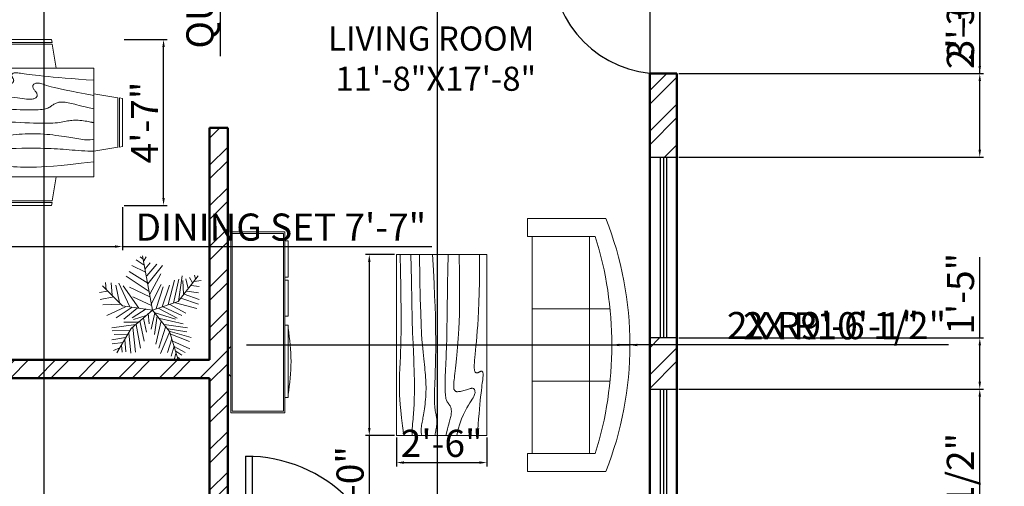
# Model space of a CAD drawing. Units: inches. Extents: x 635 to 1184, y 1837 to 2697.
# Tile 4 of 6: x 857 to 1184, y 2201 to 2356. Entities that reach past the tile are written whole.
import ezdxf

# ---------------------------------------------------------------- set-up
doc = ezdxf.new("R2010")
doc.units = ezdxf.units.IN
for name, color, linetype, lineweight in [('A-ANNO-DIMS', 2, 'Continuous', 18), ('A-AREA-IDEN', 7, 'Continuous', 25), ('A-DOOR', 4, 'Continuous', 25), ('A-FURN', 8, 'Continuous', 18), ('A-GLAZ', 244, 'Continuous', 25), ('A-WALL', 7, 'Continuous', 50), ('A-WALL-PATT', 252, 'Continuous', 13), ('L-PLNT', 94, 'Continuous', 13)]:
    doc.layers.add(name, color=color, linetype=linetype, lineweight=lineweight)
doc.styles.get("Standard").update_dxf_attribs({"font": 'arial.ttf'})
doc.dimstyles.new('ISO-25', dxfattribs={"dimtxt": 9, "dimasz": 2.5, "dimexe": 1.25, "dimexo": 0.625, "dimtad": 1, "dimlunit": 3, "dimtxsty": 'Standard', "dimcen": 2.5, "dimadec": 0, "dimazin": 0, "dimtfac": 1, "dimtmove": 0, "dimatfit": 3, "dimfxl": 1, "dimarcsym": 0})

# ---------------------------------------------------------------- blocks, each defined once
blk = doc.blocks.new('*U3')
for p, q in [((0, 0), (0, -6)), ((40, 0), (40, -6))]:
    blk.add_line(p, q)
blk.add_lwpolyline([(0, 0), (0, 40), (1.75, 40), (1.75, 0)], close=True)
blk.add_arc((0, 0), 40, 0, 90)
blk = doc.blocks.new('*U4')
for p, q in [((0, 0), (0, -6)), ((-40, 0), (-40, -6))]:
    blk.add_line(p, q)
blk.add_lwpolyline([(0, 0), (0, 40), (-1.75, 40), (-1.75, 0)], close=True)
blk.add_arc((0, 0), 40, 90, 180)
blk = doc.blocks.new('Dining Set - 36 x 72 in.')
for p, q in [((-22, 27.5), (-22.1562, 26.50042)), ((-5.8416, 26.5), (-22.1534, 26.5)), ((-22, 27.5), (-6, 27.5)), ((-5.8437, 26.49966), (-6, 27.5)), ((6, 27.5), (5.8438, 26.50042)), ((22.1584, 26.5), (5.8466, 26.5)), ((6, 27.5), (22, 27.5)), ((22.1563, 26.49966), (22, 27.5)), ((-22.2343, 26.00059), (-23.4847, 17.99762)), ((-22.2304, 26), (-5.7608, 26)), ((-4.5152, 17.99762), (-5.7655, 25.99926)), ((5.7657, 26.00059), (4.5153, 17.99762)), ((5.7696, 26), (22.2392, 26)), ((23.4848, 17.99762), (22.2345, 25.99926)), ((36, 18), (-36, 18)), ((-36, 18), (-36, -18)), ((36, -18), (36, 18)), ((-45.5, 8), (-44.5004, 8.15617)), ((-45.5, 8), (-45.5, -8)), ((-44.5, -8.15843), (-44.5, 8.15338)), ((-44.0006, 8.23428), (-35.9976, 9.48474)), ((-44, 8.23041), (-44, -8.23915)), ((44.0006, 8.23428), (35.9976, 9.48474)), ((44, 8.23041), (44, -8.23915)), ((44.5, -8.15843), (44.5, 8.15338)), ((45.5, 8), (44.5005, 8.15617)), ((45.5, 8), (45.5, -8)), ((-44.4997, -8.15631), (-45.5, -8)), ((-35.9976, -9.48476), (-43.9993, -8.2345)), ((35.9976, -9.48476), (43.9993, -8.2345)), ((44.4997, -8.15631), (45.5, -8)), ((-36, -18), (36, -18)), ((-22.2343, -26.0006), (-23.4847, -17.99762)), ((-4.5152, -17.99762), (-5.7655, -25.99928)), ((5.7657, -26.0006), (4.5153, -17.99762)), ((23.4848, -17.99762), (22.2345, -25.99928)), ((-22.2304, -26), (-5.7608, -26)), ((5.7696, -26), (22.2392, -26)), ((-22, -27.5), (-22.1562, -26.50044)), ((-5.8416, -26.5), (-22.1534, -26.5)), ((-22, -27.5), (-6, -27.5)), ((-5.8437, -26.49967), (-6, -27.5)), ((6, -27.5), (5.8438, -26.50044)), ((22.1584, -26.5), (5.8466, -26.5)), ((6, -27.5), (22, -27.5)), ((22.1563, -26.49967), (22, -27.5))]:
    blk.add_line(p, q)
for points in [[(-36, 15), (-31.1772, 14.97754), (-26.8079, 14.91406), (-22.8538, 14.81543), (-19.276, 14.6875), (-16.0362, 14.53613), (-13.0957, 14.36718), (-10.4159, 14.18652), (-7.9583, 14), (-5.6904, 13.81315), (-3.6035, 13.63021), (-1.6954, 13.45508), (0.0365, 13.29166), (1.5945, 13.14388), (2.9811, 13.01562), (4.1988, 12.9108), (5.25, 12.83333), (6.1393, 12.78613), (6.8802, 12.76823), (7.4883, 12.77767), (7.9792, 12.8125), (8.3685, 12.87077), (8.6719, 12.95052), (8.9049, 13.0498), (9.0833, 13.16666), (9.2205, 13.29899), (9.3216, 13.44401), (9.3895, 13.59879), (9.4271, 13.76041), (9.4373, 13.92594), (9.4232, 14.09245), (9.3875, 14.257), (9.3333, 14.41666), (9.2638, 14.56917), (9.1836, 14.71484), (9.0975, 14.85465), (9.0104, 14.98958), (8.9272, 15.1206), (8.8529, 15.2487), (8.7922, 15.37483), (8.75, 15.5), (8.7305, 15.62467), (8.7344, 15.74739), (8.7617, 15.86621), (8.8125, 15.97916), (8.8867, 16.08431), (8.9844, 16.17968), (9.1055, 16.26334), (9.25, 16.33333), (9.4189, 16.38802), (9.6172, 16.42708), (9.8506, 16.45052), (10.125, 16.45833), (10.4463, 16.45052), (10.8203, 16.42708), (11.2529, 16.38802), (11.75, 16.33333), (12.3184, 16.26318), (12.9694, 16.17838), (13.7151, 16.07991), (14.5677, 15.96875), (15.5395, 15.84586), (16.6426, 15.71224), (17.8893, 15.56884), (19.2917, 15.41666), (20.859, 15.25667), (22.5879, 15.08984), (24.4721, 14.91715), (26.5052, 14.73958), (28.6809, 14.5581), (30.9929, 14.3737), (33.4347, 14.18733), (36, 14)], [(-36, 10), (-28.9766, 10.14274), (-23.1725, 10.20442), (-18.4241, 10.19775), (-14.5677, 10.13541), (-11.4399, 10.03011), (-8.877, 9.89453), (-6.7154, 9.74137), (-4.7917, 9.58333), (-2.9698, 9.43082), (-1.2246, 9.28515), (0.4415, 9.14534), (2.026, 9.01041), (3.5266, 8.87939), (4.9408, 8.7513), (6.266, 8.62516), (7.5, 8.5), (8.6411, 8.37549), (9.6914, 8.2539), (10.6538, 8.13818), (11.5312, 8.03125), (12.3267, 7.93603), (13.043, 7.85547), (13.6831, 7.79248), (14.25, 7.75), (14.7471, 7.7303), (15.1797, 7.73307), (15.5537, 7.75732), (15.875, 7.80208), (16.1494, 7.86637), (16.3828, 7.94922), (16.5811, 8.04964), (16.75, 8.16666), (16.8944, 8.29915), (17.0143, 8.44531), (17.1089, 8.60319), (17.1771, 8.77083), (17.218, 8.94629), (17.2305, 9.1276), (17.2137, 9.31282), (17.1667, 9.5), (17.0895, 9.6875), (16.987, 9.875), (16.8649, 10.0625), (16.7292, 10.25), (16.5856, 10.4375), (16.4401, 10.625), (16.2985, 10.8125), (16.1667, 11), (16.05, 11.18733), (15.9518, 11.3737), (15.8752, 11.5581), (15.8229, 11.73958), (15.798, 11.91715), (15.8034, 12.08984), (15.842, 12.25667), (15.9167, 12.41666), (16.0295, 12.56836), (16.1784, 12.70833), (16.3605, 12.83268), (16.5729, 12.9375), (16.8127, 13.01888), (17.0768, 13.07291), (17.3625, 13.0957), (17.6667, 13.08333), (17.9894, 13.03312), (18.3418, 12.94726), (18.7382, 12.82918), (19.1927, 12.68229), (19.7195, 12.51001), (20.3327, 12.31575), (21.0465, 12.10294), (21.875, 11.875), (22.8357, 11.63354), (23.959, 11.37304), (25.2786, 11.08618), (26.8282, 10.76562), (28.6414, 10.40405), (30.752, 9.99414), (33.1936, 9.52856), (36, 9)], [(-36, 5.5), (-30.7157, 5.3348), (-26.069, 5.20963), (-21.9946, 5.11767), (-18.4271, 5.05208), (-15.3009, 5.00602), (-12.5508, 4.97265), (-10.1112, 4.94515), (-7.9167, 4.91666), (-5.909, 4.88167), (-4.0586, 4.83984), (-2.3429, 4.79215), (-0.7396, 4.73958), (0.7739, 4.6831), (2.22, 4.6237), (3.6213, 4.56233), (5, 4.5), (6.373, 4.43782), (7.7344, 4.3776), (9.0723, 4.32129), (10.375, 4.27083), (11.6309, 4.22819), (12.8281, 4.19531), (13.9551, 4.17415), (15, 4.16666), (15.954, 4.17448), (16.819, 4.19791), (17.6001, 4.23698), (18.3021, 4.29166), (18.9299, 4.36198), (19.4883, 4.44791), (19.9823, 4.54948), (20.4167, 4.66666), (20.7969, 4.79899), (21.1302, 4.94401), (21.4245, 5.09879), (21.6875, 5.26041), (21.9271, 5.42594), (22.1511, 5.59245), (22.3672, 5.757), (22.5834, 5.91666), (22.8065, 6.06868), (23.0404, 6.21093), (23.2879, 6.34147), (23.5521, 6.45833), (23.8358, 6.55957), (24.142, 6.64323), (24.4735, 6.70735), (24.8334, 6.75), (25.2235, 6.76969), (25.642, 6.76692), (26.0858, 6.74267), (26.5521, 6.69791), (27.0379, 6.63362), (27.5404, 6.55078), (28.0565, 6.45036), (28.5834, 6.33333), (29.1242, 6.19987), (29.7071, 6.04687), (30.3661, 5.87044), (31.1354, 5.66666), (32.0493, 5.43164), (33.142, 5.16146), (34.4475, 4.85221), (36, 4.5)], [(-36, -1), (-30.7915, -0.6591), (-26.0195, -0.38216), (-21.6519, -0.16284), (-17.6563, 0.00521), (-14.0005, 0.12833), (-10.6523, 0.21289), (-7.5796, 0.26522), (-4.75, 0.29166), (-2.134, 0.29793), (0.2878, 0.28711), (2.5317, 0.26163), (4.6146, 0.22396), (6.5529, 0.17651), (8.3633, 0.12174), (10.0623, 0.06209), (11.6667, 0), (13.1899, -0.06201), (14.6341, -0.1211), (15.9982, -0.17432), (17.2813, -0.21875), (18.4823, -0.25147), (19.6003, -0.26953), (20.6343, -0.27002), (21.5834, -0.25), (22.4481, -0.20768), (23.2357, -0.14584), (23.9549, -0.06836), (24.6146, 0.02083), (25.2235, 0.11784), (25.7904, 0.21875), (26.3241, 0.31966), (26.8334, 0.41666), (27.3265, 0.50618), (27.8099, 0.58593), (28.2894, 0.65397), (28.7709, 0.70833), (29.2601, 0.74707), (29.763, 0.76823), (30.2855, 0.76985), (30.8334, 0.75), (31.4088, 0.70784), (31.9994, 0.64713), (32.589, 0.57275), (33.1615, 0.48958), (33.7008, 0.4025), (34.1908, 0.3164), (34.6153, 0.23616), (34.9584, 0.16666), (35.2099, 0.11165), (35.3848, 0.07031), (35.504, 0.04069), (35.5886, 0.02083), (35.6594, 0.00879), (35.7377, 0.0026), (35.8442, 0.00032), (36, 0)], [(-36, -6.5), (-27.1843, -6.31267), (-20.084, -6.1263), (-14.469, -5.9419), (-10.1094, -5.76042), (-6.7752, -5.58285), (-4.2363, -5.41016), (-2.2629, -5.24333), (-0.625, -5.08334), (0.8708, -4.93099), (2.2715, -4.78646), (3.5872, -4.64974), (4.8281, -4.52084), (6.0046, -4.39974), (7.127, -4.28646), (8.2053, -4.18099), (9.25, -4.08334), (10.2705, -3.99382), (11.2734, -3.91407), (12.2647, -3.84603), (13.25, -3.79167), (14.2354, -3.75293), (15.2266, -3.73177), (16.2295, -3.73015), (17.25, -3.75), (18.2912, -3.79248), (19.3451, -3.85547), (20.4009, -3.93604), (21.4479, -4.03125), (22.4754, -4.13819), (23.4727, -4.25391), (24.4289, -4.37549), (25.3334, -4.5), (26.1785, -4.62492), (26.9694, -4.74935), (27.7145, -4.87281), (28.4219, -4.99479), (29.1, -5.11483), (29.7572, -5.23242), (30.4016, -5.34709), (31.0417, -5.45834), (31.6837, -5.56437), (32.3262, -5.65821), (32.9658, -5.73153), (33.599, -5.77604), (34.2224, -5.78345), (34.8327, -5.74545), (35.4264, -5.65373), (36, -5.5)], [(-36, -10), (-26.4022, -9.81299), (-18.4675, -9.62891), (-11.9839, -9.45069), (-6.7396, -9.28125), (-2.5226, -9.12354), (0.8789, -8.98047), (3.6769, -8.85498), (6.0833, -8.75), (8.2767, -8.66765), (10.3021, -8.60677), (12.1712, -8.56543), (13.8958, -8.54167), (15.4876, -8.53353), (16.9583, -8.53907), (18.3197, -8.55632), (19.5834, -8.58334), (20.7616, -8.61841), (21.8685, -8.66081), (22.9188, -8.71004), (23.9271, -8.76563), (24.9081, -8.82707), (25.8763, -8.89388), (26.8465, -8.96558), (27.8334, -9.04167), (28.8474, -9.12118), (29.8828, -9.20117), (30.93, -9.27824), (31.9792, -9.34896), (33.0205, -9.40991), (34.0443, -9.45768), (35.0407, -9.48885), (36, -9.5)], [(-36, -14.5), (-30.0881, -14.33513), (-25.0332, -14.21224), (-20.7312, -14.12647), (-17.0781, -14.07292), (-13.97, -14.04671), (-11.3027, -14.04297), (-8.9724, -14.05681), (-6.875, -14.08334), (-4.9224, -14.11833), (-3.0905, -14.16016), (-1.3709, -14.20785), (0.2448, -14.26042), (1.7647, -14.3169), (3.1973, -14.3763), (4.5507, -14.43767), (5.8333, -14.5), (7.0554, -14.5621), (8.235, -14.62175), (9.3922, -14.67652), (10.5469, -14.72396), (11.7192, -14.76164), (12.929, -14.78711), (14.1965, -14.79794), (15.5417, -14.79167), (16.9933, -14.76424), (18.6152, -14.70508), (20.4804, -14.60197), (22.6615, -14.44271), (25.2312, -14.21509), (28.2624, -13.9069), (31.8277, -13.50594), (36, -13)]]:
    blk.add_lwpolyline(points)
blk = doc.blocks.new('Sofa - Roundback 7 ft.')
for p, q in [((-12.00002, -32.4421), (-12.00003, -6.5971)), ((11.99997, -32.4421), (11.99998, -6.5971)), ((-36.000027, -34), (-36.000027, -11.4696)), ((35.99998, -34), (35.99998, -11.4696)), ((-35.999844, -13.3819), (35.9998, -13.3819)), ((-36.000027, -32.4421), (35.99998, -32.4421))]:
    blk.add_line(p, q)
for points in [[(-36.000027, -34), (-42.000027, -34), (-42.000027, -8)], [(41.99998, -8), (41.99998, -34), (35.99998, -34)]]:
    blk.add_lwpolyline(points)
for centre, radius, start, end in [((0, -114.25), 114.25, 68.43141, 111.5686), ((-0.00001, -127.1968), 121.1968, 72.72033, 107.2797)]:
    blk.add_arc(centre, radius, start, end)
blk = doc.blocks.new('Table - Rectangular Woodgrain 60 x 30 in.')
for p, q in [((0, 0), (0, -30)), ((60, 0), (0, 0)), ((60, -30), (60, 0)), ((0, -30), (60, -30))]:
    blk.add_line(p, q)
for points in [[(0, -2.4), (4.8155, -2.418), (9.0302, -2.4688), (12.709, -2.5477), (15.9167, -2.65), (18.7181, -2.7711), (21.1781, -2.9063), (23.3616, -3.0508), (25.3333, -3.2), (27.1477, -3.3495), (28.8172, -3.4958), (30.3437, -3.636), (31.7291, -3.7667), (32.9756, -3.8849), (34.0849, -3.9875), (35.059, -4.0714), (35.9, -4.1334), (36.6114, -4.1711), (37.2041, -4.1854), (37.6906, -4.1779), (38.0833, -4.15), (38.3948, -4.1034), (38.6375, -4.0396), (38.8239, -3.9602), (38.9666, -3.8667), (39.0764, -3.7608), (39.1573, -3.6448), (39.2116, -3.521), (39.2416, -3.3917), (39.2498, -3.2593), (39.2385, -3.1261), (39.21, -2.9944), (39.1666, -2.8667), (39.111, -2.7447), (39.0468, -2.6281), (38.978, -2.5163), (38.9083, -2.4083), (38.8418, -2.3035), (38.7823, -2.201), (38.7337, -2.1001), (38.7, -2), (38.6844, -1.9003), (38.6875, -1.8021), (38.7094, -1.707), (38.75, -1.6167), (38.8094, -1.5326), (38.8875, -1.4563), (38.9844, -1.3893), (39.1, -1.3333), (39.2351, -1.2896), (39.3937, -1.2583), (39.5804, -1.2396), (39.8, -1.2333), (40.057, -1.2396), (40.3562, -1.2583), (40.7023, -1.2896), (41.1, -1.3333), (41.5547, -1.3895), (42.0755, -1.4573), (42.6721, -1.5361), (43.3542, -1.625), (44.1316, -1.7233), (45.014, -1.8302), (46.0114, -1.9449), (47.1333, -2.0667), (48.3862, -2.1947), (49.7625, -2.3281), (51.2513, -2.4663), (52.8416, -2.6083), (54.5226, -2.7535), (56.2833, -2.9011), (58.1127, -3.0501), (60, -3.2)], [(0, -9.2), (6.5759, -9.0858), (11.9385, -9.0365), (16.2527, -9.0418), (19.6833, -9.0917), (22.3952, -9.1759), (24.5531, -9.2844), (26.322, -9.4069), (27.8666, -9.5333), (29.3241, -9.6553), (30.7203, -9.7719), (32.0532, -9.8837), (33.3208, -9.9917), (34.5213, -10.0965), (35.6526, -10.199), (36.7128, -10.2999), (37.7, -10.4), (38.6129, -10.4996), (39.4531, -10.5969), (40.223, -10.6895), (40.925, -10.775), (41.5613, -10.8512), (42.1344, -10.9156), (42.6465, -10.966), (43.1, -11), (43.4976, -11.0158), (43.8437, -11.0136), (44.143, -10.9942), (44.4, -10.9583), (44.6195, -10.9069), (44.8062, -10.8406), (44.9648, -10.7603), (45.1, -10.6667), (45.2155, -10.5598), (45.3114, -10.4365), (45.3871, -10.2929), (45.4416, -10.125), (45.4743, -9.929), (45.4844, -9.7011), (45.4709, -9.4371), (45.4333, -9.1333), (45.3716, -8.7883), (45.2896, -8.4104), (45.1919, -8.0107), (45.0833, -7.6), (44.9685, -7.1893), (44.8521, -6.7896), (44.7388, -6.4117), (44.6333, -6.0667), (44.54, -5.7628), (44.4614, -5.4979), (44.4001, -5.2675), (44.3583, -5.0667), (44.3384, -4.8909), (44.3427, -4.7354), (44.3736, -4.5956), (44.4333, -4.4667), (44.5236, -4.3453), (44.6427, -4.2333), (44.7884, -4.1339), (44.9583, -4.05), (45.1501, -3.9849), (45.3614, -3.9417), (45.59, -3.9234), (45.8333, -3.9333), (46.0915, -3.9749), (46.3734, -4.0531), (46.6906, -4.1736), (47.0542, -4.3417), (47.4756, -4.5629), (47.9661, -4.8427), (48.5372, -5.1866), (49.2, -5.6), (49.9676, -6.0844), (50.8594, -6.625), (51.8965, -7.2031), (53.1, -7.8), (54.491, -8.3969), (56.0906, -8.975), (57.9199, -9.5156), (60, -10)], [(0, -12.8), (5.1847, -12.9322), (9.6213, -13.0323), (13.3963, -13.1059), (16.5958, -13.1583), (19.3063, -13.1952), (21.614, -13.2219), (23.6054, -13.2439), (25.3666, -13.2667), (26.9728, -13.2947), (28.4531, -13.3281), (29.8256, -13.3663), (31.1083, -13.4083), (32.3191, -13.4535), (33.476, -13.501), (34.597, -13.5501), (35.7, -13.6), (36.7984, -13.6497), (37.8875, -13.6979), (38.9578, -13.743), (40, -13.7833), (41.0047, -13.8174), (41.9625, -13.8438), (42.864, -13.8607), (43.7, -13.8667), (44.4631, -13.8604), (45.1552, -13.8417), (45.7801, -13.8104), (46.3416, -13.7667), (46.8439, -13.7104), (47.2906, -13.6417), (47.6858, -13.5604), (48.0333, -13.4667), (48.3375, -13.3608), (48.6042, -13.2448), (48.8396, -13.121), (49.05, -12.9917), (49.2417, -12.8593), (49.4208, -12.7261), (49.5937, -12.5944), (49.7667, -12.4667), (49.9452, -12.3451), (50.1323, -12.2313), (50.3303, -12.1268), (50.5416, -12.0333), (50.7686, -11.9524), (51.0135, -11.8854), (51.2788, -11.8341), (51.5666, -11.8), (51.8785, -11.7843), (52.2116, -11.7865), (52.562, -11.8059), (52.926, -11.8417), (53.2998, -11.8931), (53.6795, -11.9594), (54.0614, -12.0397), (54.4416, -12.1333), (54.8223, -12.2401), (55.2293, -12.3625), (55.6942, -12.5037), (56.2489, -12.6667), (56.9251, -12.8547), (57.7545, -13.0708), (58.7689, -13.3182), (60, -13.6)], [(0, -18), (5.124, -17.7273), (9.6609, -17.5057), (13.6705, -17.3303), (17.2125, -17.1958), (20.3467, -17.0973), (23.1328, -17.0297), (25.6307, -16.9878), (27.9, -16.9667), (29.9928, -16.9617), (31.9302, -16.9703), (33.7254, -16.9907), (35.3917, -17.0208), (36.9423, -17.0588), (38.3906, -17.1026), (39.7499, -17.1503), (41.0333, -17.2), (42.2519, -17.2496), (43.4073, -17.2969), (44.4986, -17.3395), (45.525, -17.375), (46.4858, -17.4012), (47.3802, -17.4156), (48.2074, -17.416), (48.9667, -17.4), (49.6583, -17.3662), (50.2872, -17.3167), (50.8595, -17.2547), (51.3812, -17.1833), (51.8584, -17.1057), (52.2971, -17.025), (52.7034, -16.9443), (53.0833, -16.8667), (53.443, -16.7951), (53.789, -16.7313), (54.128, -16.6768), (54.4666, -16.6334), (54.8115, -16.6024), (55.1693, -16.5854), (55.5465, -16.5841), (55.95, -16.6), (56.3828, -16.6337), (56.8346, -16.6823), (57.2915, -16.7418), (57.7396, -16.8084), (58.165, -16.878), (58.5539, -16.9469), (58.8924, -17.0111), (59.1666, -17.0667), (59.3679, -17.1107), (59.5078, -17.1438), (59.6032, -17.1675), (59.6708, -17.1833), (59.7275, -17.193), (59.7901, -17.1979), (59.8753, -17.1998), (60, -17.2)], [(0, -22.4), (8.0098, -22.2501), (14.4094, -22.1011), (19.4168, -21.9535), (23.25, -21.8083), (26.1269, -21.6663), (28.2656, -21.5281), (29.884, -21.3947), (31.2, -21.2667), (32.3967, -21.1448), (33.5172, -21.0292), (34.5697, -20.9198), (35.5625, -20.8167), (36.5037, -20.7198), (37.4015, -20.6292), (38.2642, -20.5448), (39.1, -20.4667), (39.9164, -20.3951), (40.7187, -20.3313), (41.5117, -20.2768), (42.3, -20.2333), (43.0883, -20.2024), (43.8812, -20.1854), (44.6836, -20.1841), (45.5, -20.2), (46.3328, -20.234), (47.1747, -20.2844), (48.0163, -20.3488), (48.8479, -20.425), (49.66, -20.5106), (50.4429, -20.6031), (51.1872, -20.7004), (51.8833, -20.8), (52.5246, -20.8999), (53.1166, -20.9995), (53.6681, -21.0983), (54.1875, -21.1958), (54.6834, -21.2919), (55.1646, -21.3859), (55.6394, -21.4777), (56.1167, -21.5667), (56.6028, -21.6515), (57.0961, -21.7266), (57.5929, -21.7852), (58.0896, -21.8208), (58.5823, -21.8268), (59.0674, -21.7964), (59.5412, -21.723), (60, -21.6)], [(0, -25.2), (8.6355, -25.0504), (15.7026, -24.9031), (21.4049, -24.7606), (25.9458, -24.625), (29.529, -24.4988), (32.3578, -24.3844), (34.6359, -24.284), (36.5667, -24.2), (38.3213, -24.1341), (39.9417, -24.0854), (41.437, -24.0523), (42.8167, -24.0333), (44.0901, -24.0268), (45.2667, -24.0313), (46.3557, -24.0451), (47.3667, -24.0667), (48.309, -24.0947), (49.1928, -24.1287), (50.0284, -24.168), (50.826, -24.2125), (51.5959, -24.2617), (52.3483, -24.3151), (53.0935, -24.3725), (53.8417, -24.4334), (54.6009, -24.497), (55.3699, -24.561), (56.1454, -24.6226), (56.9239, -24.6792), (57.7021, -24.7279), (58.4764, -24.7662), (59.2435, -24.7911), (60, -24.8)], [(0, -28.8), (5.6867, -28.6681), (10.45, -28.5698), (14.407, -28.5012), (17.675, -28.4584), (20.3711, -28.4374), (22.6125, -28.4344), (24.5164, -28.4455), (26.2, -28.4667), (27.762, -28.4947), (29.2276, -28.5281), (30.6033, -28.5663), (31.8958, -28.6084), (33.1118, -28.6535), (34.2578, -28.7011), (35.3405, -28.7501), (36.3666, -28.8), (37.3443, -28.8497), (38.288, -28.8974), (39.2137, -28.9412), (40.1375, -28.9792), (41.0753, -29.0093), (42.0432, -29.0297), (43.0572, -29.0384), (44.1333, -29.0333), (45.2936, -29.0114), (46.5843, -28.9641), (48.0579, -28.8816), (49.7666, -28.7542), (51.7629, -28.5721), (54.0989, -28.3255), (56.8272, -28.0048), (60, -27.6)]]:
    blk.add_lwpolyline(points)
blk = doc.blocks.new('Entertainment Center')
for p, q in [((-4, 0), (-5, -1)), ((4, 0), (-4, 0)), ((5, -1), (4, 0)), ((-17, -19), (-17, -1)), ((-17, -1), (43, -1)), ((-16.5, -18.5), (-16.5, -1.5)), ((-16.5, -1.5), (42.5, -1.5)), ((42.5, -1.5), (42.5, -18.5)), ((43, -1), (43, -19)), ((43, -19), (-17, -19)), ((42.5, -18.5), (-16.5, -18.5)), ((-12, -20), (-12, -19)), ((12, -19), (12, -20)), ((15, -20), (15, -19)), ((27, -19), (27, -20)), ((28, -20), (28, -19)), ((40, -19), (40, -20)), ((12, -20), (-12, -20)), ((27, -20), (15, -20)), ((40, -20), (28, -20))]:
    blk.add_line(p, q)
blk.add_arc((0, 40), 61, 259.6111, 280.3889)
blk = doc.blocks.new('*U15')
for p, q in [((-8.737, 47.138), (-17.069, 52.711)), ((-10.186, 53.64), (-13.084, 55.962)), ((0, 0), (-10.5, 57)), ((-9.099, 51.782), (-6.563, 55.962)), ((-7.288, 39.707), (-21.778, 46.673)), ((-7.65, 43.423), (-2.578, 49.46)), ((-5.839, 35.992), (4.667, 48.067)), ((-5.114, 27.632), (10.463, 46.673)), ((-3.665, 19.273), (-27.574, 35.527)), ((-5.114, 28.097), (-24.676, 40.636)), ((-2.941, 16.486), (8.652, 37.85)), ((16.259, 5.805), (23.142, 31.348)), ((22.055, 7.198), (27.489, 32.277)), ((27, 9), (48, 36)), ((27.127, 9.056), (31.112, 35.992)), ((35.096, 32.741), (37.27, 22.524)), ((38.719, 34.134), (41.979, 28.561)), ((44.153, 36.456), (45.239, 32.741)), ((-31.5, 4.5), (-52.5, 25.5)), ((-48.585, 21.131), (-49.309, 29.026)), ((-43.513, 28.561), (-42.427, 15.558)), ((-38.442, 26.239), (-34.819, 7.663)), ((-35.544, 28.097), (-24.314, 3.947)), ((-14.533, 2.09), (-30.834, 25.31)), ((-24.314, 23.917), (-2.941, 13.7)), ((-1.129, 6.734), (9.014, 26.704)), ((3.942, 1.625), (11.187, 24.381)), ((10.101, 3.483), (17.708, 26.239)), ((31.836, 30.883), (32.561, 16.486)), ((40.53, 25.775), (48.862, 24.846)), ((43.791, 29.954), (51.036, 30.883)), ((-47.498, 19.737), (-55.83, 18.344)), ((-40.615, 13.7), (-55.105, 10.913)), ((-20.691, 13.7), (-1.129, 4.876)), ((29.662, 12.307), (48.137, 6.269)), ((33.285, 16.486), (48.862, 10.913)), ((36.183, 19.737), (48.137, 17.88)), ((-33.37, 6.269), (-52.207, 5.34)), ((-28.299, 3.483), (-47.86, -5.805)), ((-21.416, 3.018), (-38.079, -8.128)), ((0, 0), (-31.5, 4.5)), ((-15.982, 2.09), (-30.11, -9.521)), ((0, 0), (-22.5, -19.5)), ((-6.563, 1.161), (-21.416, -8.128)), ((0, 0), (27, 9)), ((0, 0), (18, -22.5)), ((6.478, 1.625), (26.04, -8.592)), ((11.187, 3.483), (30.749, -5.805)), ((18.07, 5.805), (35.096, -3.483)), ((24.229, 7.663), (46.688, 1.625)), ((-6.563, -5.805), (-19.967, -9.985)), ((-9.461, -8.592), (-6.201, -23.453)), ((-4.752, -3.483), (-3.665, -14.629)), ((2.493, -3.019), (-1.491, -20.202)), ((1.769, -2.555), (24.229, -9.521)), ((5.029, -6.27), (2.131, -25.775)), ((7.565, -9.056), (32.198, -14.629)), ((-17.431, -15.094), (-42.789, -18.809)), ((-22.5, -19.5), (-37.5, -45)), ((-15.257, -12.772), (-30.11, -12.772)), ((-20.691, -18.345), (-17.793, -44.352)), ((-17.069, -15.094), (-12.721, -40.172)), ((-13.446, -11.378), (-8.737, -32.741)), ((9.014, -11.378), (3.58, -35.992)), ((14.085, -16.951), (6.478, -40.172)), ((12.274, -15.094), (36.907, -18.809)), ((16.259, -19.738), (36.183, -22.989)), ((-28.299, -29.026), (-42.789, -31.348)), ((-24.314, -21.596), (-42.427, -22.06)), ((-26.849, -26.24), (-40.253, -25.775)), ((-29.023, -30.884), (-27.936, -43.887)), ((-25.038, -23.918), (-22.865, -45.281)), ((18.07, -22.524), (8.289, -45.745)), ((20.244, -30.419), (15.897, -44.816)), ((18, -22.5), (27, -52.5)), ((18.433, -22.524), (40.53, -29.026)), ((19.157, -25.311), (38.719, -33.206)), ((-30.834, -34.135), (-42.427, -35.528)), ((-34.457, -39.708), (-40.978, -42.494)), ((-32.646, -36.921), (-31.921, -44.352)), ((22.78, -37.85), (19.519, -48.532)), ((21.331, -32.741), (39.081, -40.636)), ((22.78, -38.314), (34.372, -44.816)), ((24.591, -45.745), (23.142, -50.854)), ((24.591, -43.423), (30.749, -47.603)), ((26.764, -49.925), (28.213, -50.854))]:
    blk.add_line(p, q)
blk = doc.blocks.new('WIN-60IN')
for p, q in [((0, 5.5), (60, 5.5)), ((0, 4.5), (60, 4.5)), ((0, 3.5), (60, 3.5))]:
    blk.add_line(p, q)
blk.add_lwpolyline([(0, 9), (60, 9), (60, 0), (0, 0)], close=True)
blk = doc.blocks.new('*D35')
at = {"layer": 'A-ANNO-DIMS', "color": 0, "lineweight": -2, "transparency": 16777216}
for p, q in [((935.16, 2529.14), (922.53, 2529.14)), ((923.78, 2526.64), (923.78, 2451.64)), ((935.16, 2449.14), (922.53, 2449.14)), ((923.78, 2449.14), (923.78, 2343.94))]:
    blk.add_line(p, q, dxfattribs=at)
at = {"layer": 'A-ANNO-DIMS', "color": 0, "transparency": 16777216}
for points in [[(923.37, 2526.64), (924.2, 2526.64), (923.78, 2529.14)], [(923.37, 2451.64), (924.2, 2451.64), (923.78, 2449.14)]]:
    blk.add_solid(points, dxfattribs=at)
at = {"layer": 'DEFPOINTS', "color": 0, "transparency": 16777216}
for p in [(935.78, 2529.14), (923.78, 2449.14), (935.78, 2449.14)]:
    blk.add_point(p, dxfattribs=at)
at = {"layer": 'A-ANNO-DIMS', "color": 0, "transparency": 16777216, "insert": (918.23, 2395.29), "char_height": 9, "attachment_point": 5, "rotation": 90}
blk.add_mtext('QUEEN BED 6\'-8"', dxfattribs=at)
blk = doc.blocks.new('*D37')
at = {"layer": 'A-ANNO-DIMS', "color": 0, "lineweight": -2, "transparency": 16777216}
for p, q in [((800.35, 2293.79), (800.35, 2279.52)), ((891.35, 2293.79), (891.35, 2279.52)), ((802.85, 2280.77), (888.85, 2280.77)), ((891.35, 2280.77), (994.02, 2280.77))]:
    blk.add_line(p, q, dxfattribs=at)
at = {"layer": 'A-ANNO-DIMS', "color": 0, "transparency": 16777216}
for points in [[(802.85, 2281.18), (802.85, 2280.35), (800.35, 2280.77)], [(888.85, 2281.18), (888.85, 2280.35), (891.35, 2280.77)]]:
    blk.add_solid(points, dxfattribs=at)
at = {"layer": 'DEFPOINTS', "color": 0, "transparency": 16777216}
for p in [(800.35, 2294.42), (891.35, 2294.42), (891.35, 2280.77)]:
    blk.add_point(p, dxfattribs=at)
at = {"layer": 'A-ANNO-DIMS', "color": 0, "transparency": 16777216, "insert": (943.93, 2286.05), "char_height": 9, "attachment_point": 5}
blk.add_mtext('DINING SET 7\'-7"', dxfattribs=at)
blk = doc.blocks.new('*D38')
at = {"layer": 'A-ANNO-DIMS', "color": 0, "lineweight": -2, "transparency": 16777216}
for p, q in [((891.97, 2349.42), (906.25, 2349.42)), ((905, 2296.92), (905, 2346.92)), ((891.97, 2294.42), (906.25, 2294.42))]:
    blk.add_line(p, q, dxfattribs=at)
at = {"layer": 'A-ANNO-DIMS', "color": 0, "transparency": 16777216}
for points in [[(904.58, 2346.92), (905.41, 2346.92), (905, 2349.42)], [(904.58, 2296.92), (905.41, 2296.92), (905, 2294.42)]]:
    blk.add_solid(points, dxfattribs=at)
at = {"layer": 'DEFPOINTS', "color": 0, "transparency": 16777216}
for p in [(891.35, 2349.42), (905, 2349.42), (891.35, 2294.42)]:
    blk.add_point(p, dxfattribs=at)
at = {"layer": 'A-ANNO-DIMS', "color": 0, "transparency": 16777216, "insert": (899.87, 2321.92), "char_height": 9, "attachment_point": 5, "rotation": 90}
blk.add_mtext('4\'-7"', dxfattribs=at)
blk = doc.blocks.new('*D39')
at = {"layer": 'A-ANNO-DIMS', "color": 0, "lineweight": -2, "transparency": 16777216}
for p, q in [((981.62, 2278.1), (972, 2278.1)), ((973.25, 2275.6), (973.25, 2220.6)), ((981.62, 2218.1), (972, 2218.1)), ((973.25, 2218.1), (973.25, 2146.87))]:
    blk.add_line(p, q, dxfattribs=at)
at = {"layer": 'A-ANNO-DIMS', "color": 0, "transparency": 16777216}
for points in [[(972.83, 2275.6), (973.67, 2275.6), (973.25, 2278.1)], [(972.83, 2220.6), (973.67, 2220.6), (973.25, 2218.1)]]:
    blk.add_solid(points, dxfattribs=at)
at = {"layer": 'DEFPOINTS', "color": 0, "transparency": 16777216}
for p in [(982.25, 2278.1), (973.25, 2218.1), (982.25, 2218.1)]:
    blk.add_point(p, dxfattribs=at)
at = {"layer": 'A-ANNO-DIMS', "color": 0, "transparency": 16777216, "insert": (968.03, 2181.23), "char_height": 9, "attachment_point": 5, "rotation": 90}
blk.add_mtext('TABLE 5\'-0"', dxfattribs=at)
blk = doc.blocks.new('*D40')
at = {"layer": 'A-ANNO-DIMS', "color": 0, "lineweight": -2, "transparency": 16777216}
for p, q in [((982.25, 2217.47), (982.25, 2207.85)), ((1012.25, 2217.47), (1012.25, 2207.85)), ((984.75, 2209.1), (1009.75, 2209.1))]:
    blk.add_line(p, q, dxfattribs=at)
at = {"layer": 'A-ANNO-DIMS', "color": 0, "transparency": 16777216}
for points in [[(984.75, 2209.51), (984.75, 2208.68), (982.25, 2209.1)], [(1009.75, 2209.51), (1009.75, 2208.68), (1012.25, 2209.1)]]:
    blk.add_solid(points, dxfattribs=at)
at = {"layer": 'DEFPOINTS', "color": 0, "transparency": 16777216}
for p in [(982.25, 2218.1), (1012.25, 2218.1), (1012.25, 2209.1)]:
    blk.add_point(p, dxfattribs=at)
at = {"layer": 'A-ANNO-DIMS', "color": 0, "transparency": 16777216, "insert": (997.25, 2214.32), "char_height": 9, "attachment_point": 5}
blk.add_mtext('2\'-6"', dxfattribs=at)
blk = doc.blocks.new('*D51')
at = {"layer": 'A-ANNO-DIMS', "color": 0, "lineweight": -2, "transparency": 16777216}
for p, q in [((1075.91, 2374.14), (1176.99, 2374.14)), ((1175.74, 2371.64), (1175.74, 2340.64)), ((1075.91, 2338.14), (1176.99, 2338.14))]:
    blk.add_line(p, q, dxfattribs=at)
at = {"layer": 'A-ANNO-DIMS', "color": 0, "transparency": 16777216}
for points in [[(1175.32, 2371.64), (1176.15, 2371.64), (1175.74, 2374.14)], [(1175.32, 2340.64), (1176.15, 2340.64), (1175.74, 2338.14)]]:
    blk.add_solid(points, dxfattribs=at)
at = {"layer": 'DEFPOINTS', "color": 0, "transparency": 16777216}
for p in [(1075.28, 2374.14), (1075.28, 2338.14), (1175.74, 2338.14)]:
    blk.add_point(p, dxfattribs=at)
at = {"layer": 'A-ANNO-DIMS', "color": 0, "transparency": 16777216, "insert": (1170.51, 2356.14), "char_height": 9, "attachment_point": 5, "rotation": 90}
blk.add_mtext('3\'-0"', dxfattribs=at)
blk = doc.blocks.new('*D52')
at = {"layer": 'A-ANNO-DIMS', "color": 0, "lineweight": -2, "transparency": 16777216}
for p, q in [((1075.91, 2233.44), (1176.99, 2233.44)), ((1175.74, 2158.64), (1175.74, 2230.94)), ((1075.91, 2156.14), (1176.99, 2156.14))]:
    blk.add_line(p, q, dxfattribs=at)
at = {"layer": 'A-ANNO-DIMS', "color": 0, "transparency": 16777216}
for points in [[(1175.32, 2230.94), (1176.15, 2230.94), (1175.74, 2233.44)], [(1175.32, 2158.64), (1176.15, 2158.64), (1175.74, 2156.14)]]:
    blk.add_solid(points, dxfattribs=at)
at = {"layer": 'DEFPOINTS', "color": 0, "transparency": 16777216}
for p in [(1075.28, 2233.44), (1175.74, 2233.44), (1075.28, 2156.14)]:
    blk.add_point(p, dxfattribs=at)
at = {"layer": 'A-ANNO-DIMS', "color": 0, "transparency": 16777216, "insert": (1170.46, 2194.79), "char_height": 9, "attachment_point": 5, "rotation": 90}
blk.add_mtext('6\'-5 1/2"', dxfattribs=at)
blk = doc.blocks.new('*D53')
at = {"layer": 'A-ANNO-DIMS', "color": 0, "lineweight": -2, "transparency": 16777216}
for p, q in [((1175.74, 2250.44), (1175.74, 2277.27)), ((1075.91, 2250.44), (1176.99, 2250.44)), ((1175.74, 2235.94), (1175.74, 2247.94)), ((1075.91, 2233.44), (1176.99, 2233.44))]:
    blk.add_line(p, q, dxfattribs=at)
at = {"layer": 'A-ANNO-DIMS', "color": 0, "transparency": 16777216}
for points in [[(1175.32, 2247.94), (1176.15, 2247.94), (1175.74, 2250.44)], [(1175.32, 2235.94), (1176.15, 2235.94), (1175.74, 2233.44)]]:
    blk.add_solid(points, dxfattribs=at)
at = {"layer": 'DEFPOINTS', "color": 0, "transparency": 16777216}
for p in [(1075.28, 2250.44), (1175.74, 2250.44), (1075.28, 2233.44)]:
    blk.add_point(p, dxfattribs=at)
at = {"layer": 'A-ANNO-DIMS', "color": 0, "transparency": 16777216, "insert": (1170.52, 2265.11), "char_height": 9, "attachment_point": 5, "rotation": 90}
blk.add_mtext('1\'-5"', dxfattribs=at)
blk = doc.blocks.new('*D54')
at = {"layer": 'A-ANNO-DIMS', "color": 0, "lineweight": -2, "transparency": 16777216}
for p, q in [((1175.74, 2338.14), (1175.74, 2386.94)), ((1075.91, 2338.14), (1176.99, 2338.14)), ((1175.74, 2312.94), (1175.74, 2335.64)), ((1075.91, 2310.44), (1176.99, 2310.44))]:
    blk.add_line(p, q, dxfattribs=at)
at = {"layer": 'A-ANNO-DIMS', "color": 0, "transparency": 16777216}
for points in [[(1175.32, 2335.64), (1176.15, 2335.64), (1175.74, 2338.14)], [(1175.32, 2312.94), (1176.15, 2312.94), (1175.74, 2310.44)]]:
    blk.add_solid(points, dxfattribs=at)
at = {"layer": 'DEFPOINTS', "color": 0, "transparency": 16777216}
for p in [(1075.28, 2338.14), (1175.74, 2338.14), (1075.28, 2310.44)]:
    blk.add_point(p, dxfattribs=at)
at = {"layer": 'A-ANNO-DIMS', "color": 0, "transparency": 16777216, "insert": (1170.46, 2363.79), "char_height": 9, "attachment_point": 5, "rotation": 90}
blk.add_mtext('2\'-3 1/2"', dxfattribs=at)
blk = doc.blocks.new('*D62')
at = {"layer": 'A-ANNO-DIMS', "color": 0, "lineweight": -2, "transparency": 16777216}
for p, q in [((829.28, 2442.52), (829.28, 1843.99)), ((865.28, 2442.52), (865.28, 1843.99)), ((831.78, 1845.24), (862.78, 1845.24))]:
    blk.add_line(p, q, dxfattribs=at)
at = {"layer": 'A-ANNO-DIMS', "color": 0, "transparency": 16777216}
for points in [[(831.78, 1845.65), (831.78, 1844.82), (829.28, 1845.24)], [(862.78, 1845.65), (862.78, 1844.82), (865.28, 1845.24)]]:
    blk.add_solid(points, dxfattribs=at)
at = {"layer": 'DEFPOINTS', "color": 0, "transparency": 16777216}
for p in [(829.28, 2443.14), (865.28, 2443.14), (865.28, 1845.24)]:
    blk.add_point(p, dxfattribs=at)
at = {"layer": 'A-ANNO-DIMS', "color": 0, "transparency": 16777216, "insert": (847.28, 1850.46), "char_height": 9, "attachment_point": 5}
blk.add_mtext('3\'-0"', dxfattribs=at)
blk = doc.blocks.new('*D63')
at = {"layer": 'A-ANNO-DIMS', "color": 0, "lineweight": -2, "transparency": 16777216}
for p, q in [((995.78, 2448.52), (995.78, 1843.99)), ((1066.28, 2448.52), (1066.28, 1843.99)), ((998.28, 1845.24), (1063.78, 1845.24))]:
    blk.add_line(p, q, dxfattribs=at)
at = {"layer": 'A-ANNO-DIMS', "color": 0, "transparency": 16777216}
for points in [[(998.28, 1845.65), (998.28, 1844.82), (995.78, 1845.24)], [(1063.78, 1845.65), (1063.78, 1844.82), (1066.28, 1845.24)]]:
    blk.add_solid(points, dxfattribs=at)
at = {"layer": 'DEFPOINTS', "color": 0, "transparency": 16777216}
for p in [(995.78, 2449.14), (1066.28, 2449.14), (1066.28, 1845.24)]:
    blk.add_point(p, dxfattribs=at)
at = {"layer": 'A-ANNO-DIMS', "color": 0, "transparency": 16777216, "insert": (1031.03, 1850.52), "char_height": 9, "attachment_point": 5}
blk.add_mtext('5\'-10 1/2"', dxfattribs=at)
blk = doc.blocks.new('*D64')
at = {"layer": 'A-ANNO-DIMS', "color": 0, "lineweight": -2, "transparency": 16777216}
for p, q in [((932.49, 2248.11), (1053.69, 2248.11)), ((1156.55, 2248.11), (1056.19, 2248.11))]:
    blk.add_line(p, q, dxfattribs=at)
at = {"layer": 'A-ANNO-DIMS', "color": 0, "transparency": 16777216}
blk.add_solid([(1056.19, 2248.53), (1056.19, 2247.7), (1053.69, 2248.11)], dxfattribs=at)
at = {"layer": 'DEFPOINTS', "color": 0, "transparency": 16777216}
for p in [(932.49, 2248.11), (1053.69, 2248.11)]:
    blk.add_point(p, dxfattribs=at)
at = {"layer": 'A-ANNO-DIMS', "color": 0, "transparency": 16777216, "insert": (1126.41, 2253.33), "char_height": 9, "attachment_point": 5, "rotation": 360}
blk.add_mtext('2X R10\'-1"', dxfattribs=at)
blk = doc.blocks.new('*D65')
at = {"layer": 'A-ANNO-DIMS', "color": 0, "lineweight": -2, "transparency": 16777216}
for p, q in [((945.44, 2248.11), (1059.69, 2248.11)), ((1165.37, 2248.11), (1062.19, 2248.11))]:
    blk.add_line(p, q, dxfattribs=at)
at = {"layer": 'A-ANNO-DIMS', "color": 0, "transparency": 16777216}
blk.add_solid([(1062.19, 2248.53), (1062.19, 2247.7), (1059.69, 2248.11)], dxfattribs=at)
at = {"layer": 'DEFPOINTS', "color": 0, "transparency": 16777216}
for p in [(945.44, 2248.11), (1059.69, 2248.11)]:
    blk.add_point(p, dxfattribs=at)
at = {"layer": 'A-ANNO-DIMS', "color": 0, "transparency": 16777216, "insert": (1128.24, 2253.39), "char_height": 9, "attachment_point": 5, "rotation": 360}
blk.add_mtext('2X R9\'-6 1/2"', dxfattribs=at)

msp = doc.modelspace()

# ---------------------------------------------------------------- hatches: boundary and pattern name
at = {"layer": 'A-WALL-PATT'}
h = msp.add_hatch(dxfattribs=at)
h.set_pattern_fill('ANSI32', color=256)
h.paths.add_polyline_path([(723.282, 2313.142), (714.282, 2313.142), (714.282, 2234.142), (718.782, 2234.142), (723.282, 2234.142), (723.282, 2237.142), (779.782, 2237.142), (779.782, 2243.142), (723.282, 2243.142)])
h.paths.add_polyline_path([(926.282, 2320.142), (920.282, 2320.142), (920.282, 2243.142), (845.782, 2243.142), (845.782, 2237.142), (920.282, 2237.142), (920.282, 2093.142), (860.282, 2093.142), (860.282, 2165.142), (854.282, 2165.142), (854.282, 2093.142), (818.782, 2093.142), (818.782, 2084.142), (929.282, 2084.142), (929.282, 2156.142), (932.282, 2156.142), (932.282, 2165.142), (926.282, 2165.142)])
h.paths.add_polyline_path([(1075.282, 2250.443), (1066.282, 2250.443), (1066.282, 2233.442), (1075.282, 2233.442)])
h.paths.add_polyline_path([(1075.282, 2173.442), (1066.282, 2173.442), (1066.282, 2165.142), (1057.782, 2165.142), (1057.782, 2156.142), (1075.282, 2156.142)])
h.paths.add_polyline_path([(997.782, 2165.142), (980.282, 2165.142), (980.282, 2156.142), (997.782, 2156.142)])
h.paths.add_polyline_path([(1075.282, 2338.142), (1066.282, 2338.142), (1066.282, 2310.443), (1075.282, 2310.443)])
h.paths.add_polyline_path([(758.782, 2093.142), (723.282, 2093.142), (723.282, 2154.642), (714.282, 2154.642), (714.282, 2084.142), (758.782, 2084.142)])
h.paths.add_polyline_path([(723.282, 2204.142), (714.282, 2204.142), (714.282, 2175.642), (723.282, 2175.642)])
h.paths.add_polyline_path([(1075.282, 2404.069), (1066.282, 2404.069), (1066.282, 2383.142), (970.282, 2383.142), (970.282, 2386.142), (964.282, 2386.142), (964.282, 2383.142), (926.282, 2383.142), (926.282, 2389.142), (920.282, 2389.142), (920.282, 2368.142), (926.282, 2368.142), (926.282, 2377.142), (1066.282, 2377.142), (1066.282, 2374.142), (1075.282, 2374.142)])
h.paths.add_polyline_path([(926.282, 2443.142), (964.282, 2443.142), (964.282, 2416.142), (970.282, 2416.142), (970.282, 2443.142), (1066.282, 2443.142), (1066.282, 2425.069), (1075.282, 2425.069), (1075.282, 2503.642), (1066.282, 2503.642), (1066.282, 2449.142), (865.282, 2449.142), (865.282, 2443.142), (920.282, 2443.142), (920.282, 2416.142), (926.282, 2416.142)])
h.paths.add_polyline_path([(829.282, 2449.142), (826.282, 2449.142), (826.282, 2527.142), (826.282, 2557.642), (820.282, 2557.642), (820.282, 2527.142), (817.282, 2527.142), (817.282, 2521.142), (820.282, 2521.142), (820.282, 2449.142), (723.282, 2449.142), (723.282, 2474.642), (714.282, 2474.642), (714.282, 2373.142), (723.282, 2373.142), (723.282, 2443.142), (829.282, 2443.142)])
h.paths.add_polyline_path([(787.282, 2527.142), (723.282, 2527.142), (723.282, 2618.142), (820.282, 2618.142), (820.282, 2587.642), (826.282, 2587.642), (826.282, 2618.142), (916.282, 2618.142), (916.282, 2627.142), (714.282, 2627.142), (714.282, 2495.642), (723.282, 2495.642), (723.282, 2521.142), (787.282, 2521.142)])
h.paths.add_polyline_path([(1075.282, 2627.142), (976.282, 2627.142), (976.282, 2618.142), (1066.282, 2618.142), (1066.282, 2563.642), (1075.282, 2563.642)])

# ---------------------------------------------------------------- linework, layer by layer
at = {"layer": 'A-WALL'}
for p, q in [((1066.282, 2338.142), (1075.282, 2338.142)), ((1066.282, 2338.142), (1066.282, 2165.142)), ((1075.282, 2338.142), (1075.282, 2156.142)), ((926.282, 2320.142), (920.282, 2320.142)), ((920.282, 2320.142), (920.282, 2243.142)), ((926.282, 2320.142), (926.282, 2165.142)), ((845.782, 2243.142), (920.282, 2243.142)), ((845.782, 2237.142), (920.282, 2237.142)), ((920.282, 2237.142), (920.282, 2093.142))]:
    msp.add_line(p, q, dxfattribs=at)

# ---------------------------------------------------------------- block references
at = {"layer": 'A-DOOR', "xscale": 0.8999999999999996, "yscale": 0.8999999999999996, "zscale": 0.8999999999999996, "rotation": 90}
msp.add_blockref('*U4', (1069.882, 2374.142), dxfattribs=at)
at = {"layer": 'A-DOOR', "xscale": 1.199999999999993, "yscale": 1.199999999999993, "zscale": 1.199999999999993}
msp.add_blockref('*U3', (932.282, 2163.225), dxfattribs=at)
at = {"layer": 'A-FURN'}
msp.add_blockref('Dining Set - 36 x 72 in.', (845.847, 2321.918), dxfattribs=at)
for name, p, rotation in [('Sofa - Roundback 7 ft.', (1059.692, 2248.114), 270), ('Entertainment Center', (926.282, 2242.642), 90), ('Table - Rectangular Woodgrain 60 x 30 in.', (1012.249, 2278.095), 270)]:
    msp.add_blockref(name, p, dxfattribs=dict(at, rotation=rotation))
at = {"layer": 'A-GLAZ', "rotation": 270.0000000000012}
for p in [(1066.282, 2310.443), (1066.282, 2233.442)]:
    msp.add_blockref('WIN-60IN', p, dxfattribs=at)
at = {"layer": 'L-PLNT', "xscale": 0.3157050638920436, "yscale": 0.3157050638920436, "zscale": 0.3157050638920436}
msp.add_blockref('*U15', (901.346, 2259.716), dxfattribs=at)

# ---------------------------------------------------------------- texts
at = {"layer": 'A-AREA-IDEN', "insert": (959.565, 2353.777), "char_height": 8, "attachment_point": 1}
msp.add_mtext_dynamic_manual_height_columns('LIVING ROOM\\P 11\'-8"X17\'-8"', width=76.11076, gutter_width=12.5, heights=[0], dxfattribs=at)

# ---------------------------------------------------------------- dimensions: what is measured, and where the dimension line sits
at = {"layer": 'A-ANNO-DIMS'}
for base, p1, p2, text, picture, middle in [((923.782, 2449.142), (935.782, 2529.142), (935.782, 2449.142), 'QUEEN BED <>', '*D35', (918.227, 2395.289)), ((973.249, 2218.095), (982.249, 2278.095), (982.249, 2218.095), 'TABLE <>', '*D39', (968.028, 2181.233))]:
    dim = msp.add_linear_dim(base=base, p1=p1, p2=p2, angle=270, text=text, dimstyle='ISO-25', override={"dimdec": 1, "dimlfac": 1, "dimrnd": 0, "dimzin": 1, "dimdsep": 46, "dimlunit": 4, "dimfrac": 2}, dxfattribs=at)
    dim.commit()
    dim.dimension.update_dxf_attribs({"geometry": picture, "text_midpoint": middle})
for base, p1, p2, picture, middle in [((1066.282, 1845.237), (995.782, 2449.142), (1066.282, 2449.142), '*D63', (1031.032, 1850.516)), ((865.282, 1845.237), (829.282, 2443.142), (865.282, 2443.142), '*D62', (847.282, 1850.461)), ((1012.249, 2209.095), (982.249, 2218.095), (1012.249, 2218.095), '*D40', (997.249, 2214.315))]:
    dim = msp.add_linear_dim(base=base, p1=p1, p2=p2, dimstyle='ISO-25', override={"dimdec": 1, "dimlfac": 1, "dimrnd": 0, "dimzin": 1, "dimdsep": 46, "dimlunit": 4, "dimfrac": 2}, dxfattribs=at)
    dim.commit()
    dim.dimension.update_dxf_attribs({"geometry": picture, "text_midpoint": middle})
for base, p1, p2, picture, middle in [((1175.738, 2338.142), (1075.282, 2310.443), (1075.282, 2338.142), '*D54', (1170.456, 2363.791)), ((1175.738, 2338.142), (1075.282, 2374.142), (1075.282, 2338.142), '*D51', (1170.515, 2356.142)), ((904.997, 2349.418), (891.347, 2294.418), (891.347, 2349.418), '*D38', (899.872, 2321.918)), ((1175.738, 2250.443), (1075.282, 2233.442), (1075.282, 2250.443), '*D53', (1170.518, 2265.107)), ((1175.738, 2233.442), (1075.282, 2156.142), (1075.282, 2233.442), '*D52', (1170.459, 2194.792))]:
    dim = msp.add_linear_dim(base=base, p1=p1, p2=p2, angle=90, dimstyle='ISO-25', override={"dimdec": 1, "dimlfac": 1, "dimrnd": 0, "dimzin": 1, "dimdsep": 46, "dimlunit": 4, "dimfrac": 2}, dxfattribs=at)
    dim.commit()
    dim.dimension.update_dxf_attribs({"geometry": picture, "text_midpoint": middle})
dim = msp.add_linear_dim(base=(891.347, 2280.768), p1=(800.347, 2294.418), p2=(891.347, 2294.418), text='DINING SET <>', dimstyle='ISO-25', override={"dimdec": 1, "dimlfac": 1, "dimrnd": 0, "dimzin": 1, "dimdsep": 46, "dimlunit": 4, "dimfrac": 2}, dxfattribs=at)
dim.commit()
dim.dimension.update_dxf_attribs({"geometry": '*D37', "text_midpoint": (943.932, 2286.046)})
for center, mpoint, picture, middle in [((945.44175, 2248.11405), (1059.69176, 2248.114), '*D65', (1128.24175, 2248.11397)), ((932.495, 2248.114), (1053.692, 2248.114), '*D64', (1126.41, 2248.114))]:
    dim = msp.add_radius_dim(center=center, mpoint=mpoint, text='2X <>', dimstyle='ISO-25', override={"dimdec": 1, "dimlfac": 1, "dimrnd": 0, "dimzin": 1, "dimdsep": 46, "dimlunit": 4, "dimfrac": 2}, dxfattribs=at)
    dim.commit()
    dim.dimension.update_dxf_attribs({"geometry": picture, "text_midpoint": middle, "dimtype": 164})

doc.saveas('drawing.dxf')
